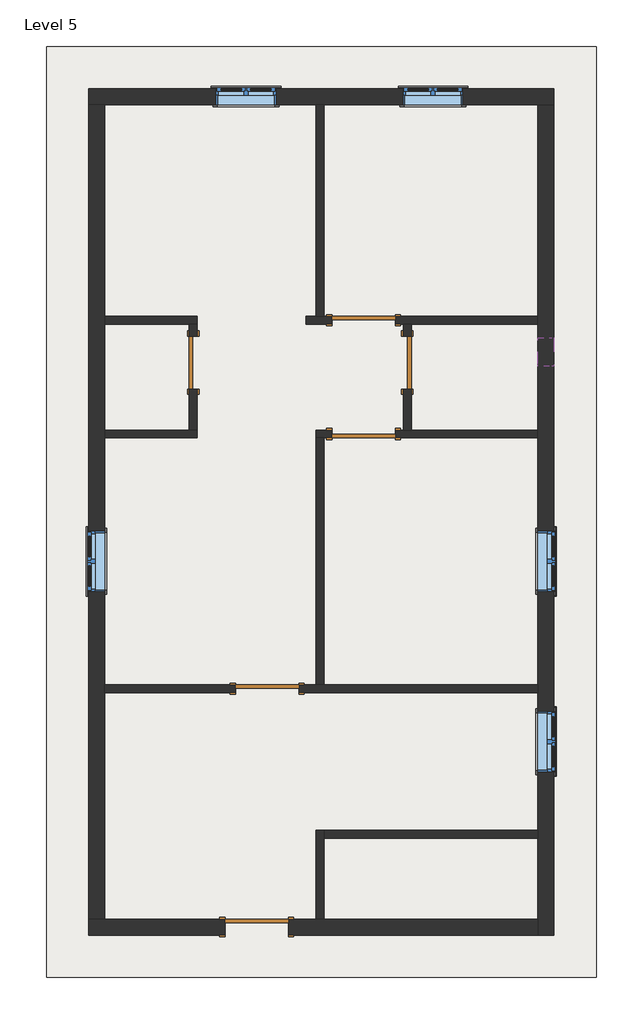
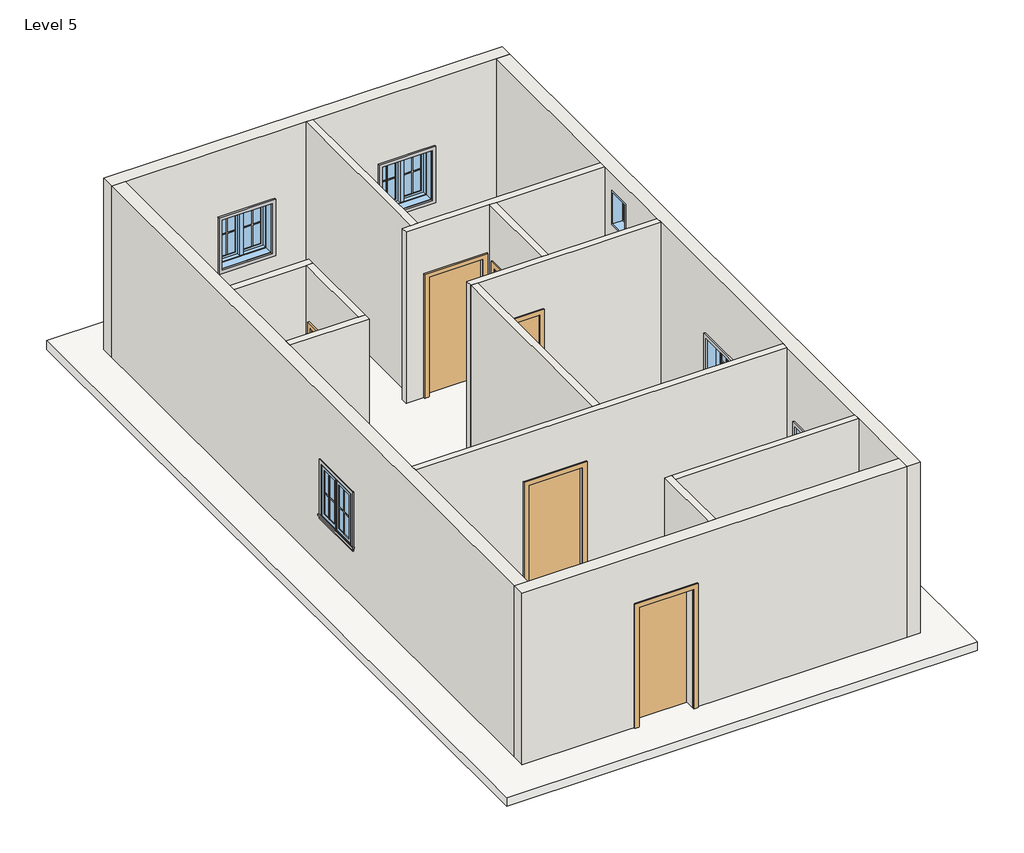
# One storey, incomplete: 20 proxies, 15 walls, 6 doors, 6 windows, 1 roof.
"""IFC4 building model written with IfcOpenShell, lengths in millimetres."""

from ifc_helpers import new_model, si_unit, frame, origin, place, context, project, spatial, polyline, outline, extrude, faceted_brep, transform, mapped, element, save
from components import muntin_pattern_2x2_muntin_pattern_2x2_b3fe6957, muntin_pattern_2x2_muntin_pattern_2x2_3e0ecaf2, trim_window_exterior_flat_with_sill_41619996, trim_window_interior_flat_picture_frame_51c85655, door_f2b275c1, door_d8f5dbb5, door_305aa2a5, door_e5f9f3c4, door_a90ba1ad, window_aa618e30, window_339605e1

model = new_model("IFC4")

# Units and contexts
model_context = context("Model", 3, world=origin())
ifc_project = project(units=[si_unit("LENGTHUNIT", "METRE", prefix="MILLI")], contexts=[model_context])

# Site, building, storey
site = spatial("IfcSite", under=ifc_project)
building = spatial("IfcBuilding", under=site)
storey = spatial("IfcBuildingStorey", under=building, Name="Level 5", Elevation=9601.2)

# Proxies
placement = place(None, origin())
muntin_pattern_2x2_muntin_pattern_2x2_shape = muntin_pattern_2x2_muntin_pattern_2x2_b3fe6957(model_context)
element("IfcBuildingElementProxy", 1, Name="Muntin Pattern_2x2 : Muntin Pattern_2x2", ObjectType="Muntin Pattern_2x2 : Muntin Pattern_2x2", at=placement, inside=storey, context=model_context, shape_type="MappedRepresentation", body=[
    mapped(muntin_pattern_2x2_muntin_pattern_2x2_shape, transform((-2560.703247, 6624.6685985, 10585.45), x_axis=(1.0, 0.0, 0.0), y_axis=(0.0, 1.0, 0.0), z_axis=(0.0, 0.0, 1.0))),
])
element("IfcBuildingElementProxy", 2, Name="Muntin Pattern_2x2 : Muntin Pattern_2x2", ObjectType="Muntin Pattern_2x2 : Muntin Pattern_2x2", at=placement, inside=storey, context=model_context, shape_type="MappedRepresentation", body=[
    mapped(muntin_pattern_2x2_muntin_pattern_2x2_shape, transform((134.871753, 6624.6685985, 10585.45), x_axis=(1.0, 0.0, 0.0), y_axis=(0.0, 1.0, 0.0), z_axis=(0.0, 0.0, 1.0))),
])
element("IfcBuildingElementProxy", 3, Name="Muntin Pattern_2x2 : Muntin Pattern_2x2", ObjectType="Muntin Pattern_2x2 : Muntin Pattern_2x2", at=placement, inside=storey, context=model_context, shape_type="MappedRepresentation", body=[
    mapped(muntin_pattern_2x2_muntin_pattern_2x2_shape, transform((2082.734253, 41.3060985, 10585.45), x_axis=(0.0, -1.0, 0.0), y_axis=(1.0, 0.0, 0.0), z_axis=(0.0, 0.0, 1.0))),
])
element("IfcBuildingElementProxy", 4, Name="Muntin Pattern_2x2 : Muntin Pattern_2x2", ObjectType="Muntin Pattern_2x2 : Muntin Pattern_2x2", at=placement, inside=storey, context=model_context, shape_type="MappedRepresentation", body=[
    mapped(muntin_pattern_2x2_muntin_pattern_2x2_shape, transform((-4603.815747, -387.3189015, 10585.45), x_axis=(0.0, 1.0, 0.0), y_axis=(-1.0, 0.0, 0.0), z_axis=(0.0, 0.0, 1.0))),
])
element("IfcBuildingElementProxy", 5, Name="Muntin Pattern_2x2 : Muntin Pattern_2x2", ObjectType="Muntin Pattern_2x2 : Muntin Pattern_2x2", at=placement, inside=storey, context=model_context, shape_type="MappedRepresentation", body=[
    mapped(muntin_pattern_2x2_muntin_pattern_2x2_shape, transform((2082.734253, -2555.8439015, 10585.45), x_axis=(0.0, -1.0, 0.0), y_axis=(1.0, 0.0, 0.0), z_axis=(0.0, 0.0, 1.0))),
])
muntin_pattern_2x2_muntin_pattern_2x2_2_shape = muntin_pattern_2x2_muntin_pattern_2x2_3e0ecaf2(model_context)
element("IfcBuildingElementProxy", 6, Name="Muntin Pattern_2x2 : Muntin Pattern_2x2", ObjectType="Muntin Pattern_2x2 : Muntin Pattern_2x2", at=placement, inside=storey, context=model_context, shape_type="MappedRepresentation", body=[
    mapped(muntin_pattern_2x2_muntin_pattern_2x2_2_shape, transform((-2132.078247, 6624.6685985, 10585.45), x_axis=(-1.0, 0.0, 0.0), y_axis=(0.0, -1.0, 0.0), z_axis=(0.0, 0.0, 1.0))),
])
element("IfcBuildingElementProxy", 7, Name="Muntin Pattern_2x2 : Muntin Pattern_2x2", ObjectType="Muntin Pattern_2x2 : Muntin Pattern_2x2", at=placement, inside=storey, context=model_context, shape_type="MappedRepresentation", body=[
    mapped(muntin_pattern_2x2_muntin_pattern_2x2_2_shape, transform((563.496753, 6624.6685985, 10585.45), x_axis=(-1.0, 0.0, 0.0), y_axis=(0.0, -1.0, 0.0), z_axis=(0.0, 0.0, 1.0))),
])
element("IfcBuildingElementProxy", 8, Name="Muntin Pattern_2x2 : Muntin Pattern_2x2", ObjectType="Muntin Pattern_2x2 : Muntin Pattern_2x2", at=placement, inside=storey, context=model_context, shape_type="MappedRepresentation", body=[
    mapped(muntin_pattern_2x2_muntin_pattern_2x2_2_shape, transform((2082.734253, -387.3189015, 10585.45), x_axis=(0.0, 1.0, 0.0), y_axis=(-1.0, 0.0, 0.0), z_axis=(0.0, 0.0, 1.0))),
])
element("IfcBuildingElementProxy", 9, Name="Muntin Pattern_2x2 : Muntin Pattern_2x2", ObjectType="Muntin Pattern_2x2 : Muntin Pattern_2x2", at=placement, inside=storey, context=model_context, shape_type="MappedRepresentation", body=[
    mapped(muntin_pattern_2x2_muntin_pattern_2x2_2_shape, transform((-4603.815747, 41.3060985, 10585.45), x_axis=(0.0, -1.0, 0.0), y_axis=(1.0, 0.0, 0.0), z_axis=(0.0, 0.0, 1.0))),
])
element("IfcBuildingElementProxy", 10, Name="Muntin Pattern_2x2 : Muntin Pattern_2x2", ObjectType="Muntin Pattern_2x2 : Muntin Pattern_2x2", at=placement, inside=storey, context=model_context, shape_type="MappedRepresentation", body=[
    mapped(muntin_pattern_2x2_muntin_pattern_2x2_2_shape, transform((2082.734253, -2984.4689015, 10585.45), x_axis=(0.0, 1.0, 0.0), y_axis=(-1.0, 0.0, 0.0), z_axis=(0.0, 0.0, 1.0))),
])
trim_window_exterior_flat_with_sill_shape = trim_window_exterior_flat_with_sill_41619996(model_context)
element("IfcBuildingElementProxy", 11, Name="Trim-Window-Exterior-Flat : with Sill", ObjectType="Trim-Window-Exterior-Flat : with Sill", at=placement, inside=storey, context=model_context, shape_type="MappedRepresentation", body=[
    mapped(trim_window_exterior_flat_with_sill_shape, transform((-2346.390747, 6634.1935985, 11430.0), x_axis=(-1.0, 0.0, 0.0), y_axis=(0.0, 0.0, 1.0), z_axis=(0.0, 1.0, 0.0))),
])
element("IfcBuildingElementProxy", 12, Name="Trim-Window-Exterior-Flat : with Sill", ObjectType="Trim-Window-Exterior-Flat : with Sill", at=placement, inside=storey, context=model_context, shape_type="MappedRepresentation", body=[
    mapped(trim_window_exterior_flat_with_sill_shape, transform((349.184253, 6634.1935985, 11430.0), x_axis=(-1.0, 0.0, 0.0), y_axis=(0.0, 0.0, 1.0), z_axis=(0.0, 1.0, 0.0))),
])
element("IfcBuildingElementProxy", 13, Name="Trim-Window-Exterior-Flat : with Sill", ObjectType="Trim-Window-Exterior-Flat : with Sill", at=placement, inside=storey, context=model_context, shape_type="MappedRepresentation", body=[
    mapped(trim_window_exterior_flat_with_sill_shape, transform((2092.259253, -173.0064015, 11430.0), x_axis=(0.0, 1.0, 0.0), y_axis=(0.0, 0.0, 1.0), z_axis=(1.0, 0.0, 0.0))),
])
element("IfcBuildingElementProxy", 14, Name="Trim-Window-Exterior-Flat : with Sill", ObjectType="Trim-Window-Exterior-Flat : with Sill", at=placement, inside=storey, context=model_context, shape_type="MappedRepresentation", body=[
    mapped(trim_window_exterior_flat_with_sill_shape, transform((-4613.340747, -173.0064015, 11430.0), x_axis=(0.0, -1.0, 0.0), y_axis=(0.0, 0.0, 1.0), z_axis=(-1.0, 0.0, 0.0))),
])
element("IfcBuildingElementProxy", 15, Name="Trim-Window-Exterior-Flat : with Sill", ObjectType="Trim-Window-Exterior-Flat : with Sill", at=placement, inside=storey, context=model_context, shape_type="MappedRepresentation", body=[
    mapped(trim_window_exterior_flat_with_sill_shape, transform((2092.259253, -2770.1564015, 11430.0), x_axis=(0.0, 1.0, 0.0), y_axis=(0.0, 0.0, 1.0), z_axis=(1.0, 0.0, 0.0))),
])
trim_window_interior_flat_picture_frame_shape = trim_window_interior_flat_picture_frame_51c85655(model_context)
element("IfcBuildingElementProxy", 16, Name="Trim-Window-Interior-Flat : Picture Frame", ObjectType="Trim-Window-Interior-Flat : Picture Frame", at=placement, inside=storey, context=model_context, shape_type="MappedRepresentation", body=[
    mapped(trim_window_interior_flat_picture_frame_shape, transform((-2346.390747, 6405.5935985, 11430.0), x_axis=(1.0, 0.0, 0.0), y_axis=(0.0, 0.0, 1.0), z_axis=(0.0, -1.0, 0.0))),
])
element("IfcBuildingElementProxy", 17, Name="Trim-Window-Interior-Flat : Picture Frame", ObjectType="Trim-Window-Interior-Flat : Picture Frame", at=placement, inside=storey, context=model_context, shape_type="MappedRepresentation", body=[
    mapped(trim_window_interior_flat_picture_frame_shape, transform((349.184253, 6405.5935985, 11430.0), x_axis=(1.0, 0.0, 0.0), y_axis=(0.0, 0.0, 1.0), z_axis=(0.0, -1.0, 0.0))),
])
element("IfcBuildingElementProxy", 18, Name="Trim-Window-Interior-Flat : Picture Frame", ObjectType="Trim-Window-Interior-Flat : Picture Frame", at=placement, inside=storey, context=model_context, shape_type="MappedRepresentation", body=[
    mapped(trim_window_interior_flat_picture_frame_shape, transform((1863.659253, -173.0064015, 11430.0), x_axis=(0.0, -1.0, 0.0), y_axis=(0.0, 0.0, 1.0), z_axis=(-1.0, 0.0, 0.0))),
])
element("IfcBuildingElementProxy", 19, Name="Trim-Window-Interior-Flat : Picture Frame", ObjectType="Trim-Window-Interior-Flat : Picture Frame", at=placement, inside=storey, context=model_context, shape_type="MappedRepresentation", body=[
    mapped(trim_window_interior_flat_picture_frame_shape, transform((-4384.740747, -173.0064015, 11430.0), x_axis=(0.0, 1.0, 0.0), y_axis=(0.0, 0.0, 1.0), z_axis=(1.0, 0.0, 0.0))),
])
element("IfcBuildingElementProxy", 20, Name="Trim-Window-Interior-Flat : Picture Frame", ObjectType="Trim-Window-Interior-Flat : Picture Frame", at=placement, inside=storey, context=model_context, shape_type="MappedRepresentation", body=[
    mapped(trim_window_interior_flat_picture_frame_shape, transform((1863.659253, -2770.1564015, 11430.0), x_axis=(0.0, -1.0, 0.0), y_axis=(0.0, 0.0, 1.0), z_axis=(-1.0, 0.0, 0.0))),
])

# Doors
door_shape = door_f2b275c1(model_context)
element("IfcDoor", 21, ObjectType="Single-Flush : 30\" x 80\"", at=placement, inside=storey, context=model_context, shape_type="MappedRepresentation", body=[
    mapped(door_shape, transform((-22.290747, 2690.8435985, 9601.2), x_axis=(0.0, 1.0, 0.0), y_axis=(-1.0, 0.0, 0.0), z_axis=(0.0, 0.0, 1.0))),
])
door_2_shape = door_d8f5dbb5(model_context)
element("IfcDoor", 22, ObjectType="Single-Flush : 30\" x 80\"", at=placement, inside=storey, context=model_context, shape_type="MappedRepresentation", body=[
    mapped(door_2_shape, transform((-3108.390747, 2690.8435985, 9601.2), x_axis=(0.0, 1.0, 0.0), y_axis=(-1.0, 0.0, 0.0), z_axis=(0.0, 0.0, 1.0))),
])
door_3_shape = door_305aa2a5(model_context)
element("IfcDoor", 23, ObjectType="Single-Flush : 36\" x 84\"", at=placement, inside=storey, context=model_context, shape_type="MappedRepresentation", body=[
    mapped(door_3_shape, transform((-650.940747, 3300.4435985, 9601.2), x_axis=(-1.0, 0.0, 0.0), y_axis=(0.0, -1.0, 0.0), z_axis=(0.0, 0.0, 1.0))),
])
door_4_shape = door_e5f9f3c4(model_context)
element("IfcDoor", 24, ObjectType="Single-Flush : 36\" x 84\"", at=placement, inside=storey, context=model_context, shape_type="MappedRepresentation", body=[
    mapped(door_4_shape, transform((-2041.590747, -2008.1564015, 9601.2), x_axis=(1.0, 0.0, 0.0), y_axis=(0.0, 1.0, 0.0), z_axis=(0.0, 0.0, 1.0))),
])
element("IfcDoor", 25, ObjectType="Single-Flush : 36\" x 84\"", at=placement, inside=storey, context=model_context, shape_type="MappedRepresentation", body=[
    mapped(door_4_shape, transform((-650.940747, 1662.1435985, 9601.2), x_axis=(-1.0, 0.0, 0.0), y_axis=(0.0, -1.0, 0.0), z_axis=(0.0, 0.0, 1.0))),
])
door_5_shape = door_a90ba1ad(model_context)
element("IfcDoor", 26, ObjectType="Single-Flush : 36\" x 84\"", at=placement, inside=storey, context=model_context, shape_type="MappedRepresentation", body=[
    mapped(door_5_shape, transform((-2193.990747, -5443.5064015, 9601.2), x_axis=(-1.0, 0.0, 0.0), y_axis=(0.0, -1.0, 0.0), z_axis=(0.0, 0.0, 1.0))),
])

# Roof
element("IfcRoof", 27, ObjectType="Generic - 12\"", at=placement, inside=storey, context=model_context, shape_type="SweptSolid", body=[
    extrude(outline(polyline([(-5222.940747, 7243.7935985), (2701.859253, 7243.7935985), (2701.859253, -6167.4064015), (-5222.940747, -6167.4064015), (-5222.940747, 7243.7935985)])), frame((0.0, 0.0, 9448.8), z_axis=(0.0, 0.0, 1.0), x_axis=(1.0, 0.0, 0.0)), (0.0, 0.0, 1.0), 152.4),
])

# Walls
element("IfcWall", 28, ObjectType="WALL4.5\"", at=placement, inside=storey, context=model_context, shape_type="Brep", body=[
    faceted_brep([(-4384.740747, 3243.2935985, 9601.2), (-3165.540747, 3243.2935985, 9601.2), (-3051.240747, 3243.2935985, 9601.2), (-3051.240747, 3243.2935985, 12649.2), (-3165.540747, 3243.2935985, 12649.2), (-4384.740747, 3243.2935985, 12649.2), (-4384.740747, 3357.5935985, 9601.2), (-4384.740747, 3357.5935985, 12649.2), (-3051.240747, 3357.5935985, 12649.2), (-3051.240747, 3357.5935985, 9601.2)], [[[0, 1, 2, 3, 4, 5]], [[6, 7, 8, 9]], [[2, 1, 0, 6, 9]], [[0, 5, 7, 6]], [[3, 2, 9, 8]], [[5, 4, 3, 8, 7]]]),
])
element("IfcWall", 29, ObjectType="WALL4.5\"", at=placement, inside=storey, context=model_context, shape_type="Brep", body=[
    faceted_brep([(-4384.740747, 1604.9935985, 9601.2), (-3051.240747, 1604.9935985, 9601.2), (-3051.240747, 1604.9935985, 12649.2), (-4384.740747, 1604.9935985, 12649.2), (-4384.740747, 1719.2935985, 9601.2), (-4384.740747, 1719.2935985, 12649.2), (-3165.540747, 1719.2935985, 12649.2), (-3051.240747, 1719.2935985, 12649.2), (-3051.240747, 1719.2935985, 9601.2), (-3165.540747, 1719.2935985, 9601.2)], [[[0, 1, 2, 3]], [[4, 5, 6, 7, 8, 9]], [[1, 0, 4, 9, 8]], [[0, 3, 5, 4]], [[2, 1, 8, 7]], [[3, 2, 7, 6, 5]]]),
])
element("IfcWall", 30, ObjectType="WALL4.5\"", at=placement, inside=storey, context=model_context, shape_type="SweptSolid", body=[
    extrude(outline(polyline([(3243.2935985, 9601.2), (3071.8435985, 9601.2), (3071.8435985, 11633.2), (2309.8435985, 11633.2), (2309.8435985, 9601.2), (1719.2935985, 9601.2), (1719.2935985, 12649.2), (3243.2935985, 12649.2), (3243.2935985, 9601.2)])), frame((-3165.540747, 0.0, 0.0), z_axis=(1.0, 0.0, 0.0), x_axis=(0.0, 1.0, 0.0)), (0.0, 0.0, 1.0), 114.3),
])
element("IfcWall", 31, ObjectType="WALL4.5\"", at=placement, inside=storey, context=model_context, shape_type="SweptSolid", body=[
    extrude(outline(polyline([(-1336.740747, 3357.5935985), (-1336.740747, 6405.5935985), (-1222.440747, 6405.5935985), (-1222.440747, 3357.5935985), (-1336.740747, 3357.5935985)])), frame((0.0, 0.0, 9601.2), z_axis=(0.0, 0.0, 1.0), x_axis=(1.0, 0.0, 0.0)), (0.0, 0.0, 1.0), 3048.0),
])
element("IfcWall", 32, ObjectType="WALL4.5\"", at=placement, inside=storey, context=model_context, shape_type="Brep", body=[
    faceted_brep([(-1481.7019184, 3243.2935985, 9601.2), (-1108.140747, 3243.2935985, 9601.2), (-1108.140747, 3243.2935985, 11734.8), (-193.740747, 3243.2935985, 11734.8), (-193.740747, 3243.2935985, 9601.2), (-79.440747, 3243.2935985, 9601.2), (34.859253, 3243.2935985, 9601.2), (1863.659253, 3243.2935985, 9601.2), (1863.659253, 3243.2935985, 12649.2), (34.859253, 3243.2935985, 12649.2), (-79.440747, 3243.2935985, 12649.2), (-1481.7019184, 3243.2935985, 12649.2), (-1108.140747, 3357.5935985, 11734.8), (-1108.140747, 3357.5935985, 9601.2), (-1222.440747, 3357.5935985, 9601.2), (-1336.740747, 3357.5935985, 9601.2), (-1481.7019184, 3357.5935985, 9601.2), (-1481.7019184, 3357.5935985, 12649.2), (-1336.740747, 3357.5935985, 12649.2), (-1222.440747, 3357.5935985, 12649.2), (1863.659253, 3357.5935985, 12649.2), (1863.659253, 3357.5935985, 9601.2), (-193.740747, 3357.5935985, 9601.2), (-193.740747, 3357.5935985, 11734.8)], [[[0, 1, 2, 3, 4, 5, 6, 7, 8, 9, 10, 11]], [[12, 13, 14, 15, 16, 17, 18, 19, 20, 21, 22, 23]], [[22, 21, 7, 6, 5, 4]], [[16, 15, 14, 13, 1, 0]], [[0, 11, 17, 16]], [[8, 7, 21, 20]], [[2, 1, 13, 12]], [[3, 2, 12, 23]], [[4, 3, 23, 22]], [[11, 10, 9, 8, 20, 19, 18, 17]]]),
])
element("IfcWall", 33, ObjectType="WALL4.5\"", at=placement, inside=storey, context=model_context, shape_type="SweptSolid", body=[
    extrude(outline(polyline([(3243.2935985, 9601.2), (3071.8435985, 9601.2), (3071.8435985, 11633.2), (2309.8435985, 11633.2), (2309.8435985, 9601.2), (1719.2935985, 9601.2), (1719.2935985, 12649.2), (3243.2935985, 12649.2), (3243.2935985, 9601.2)])), frame((-79.440747, 0.0, 0.0), z_axis=(1.0, 0.0, 0.0), x_axis=(0.0, 1.0, 0.0)), (0.0, 0.0, 1.0), 114.3),
])
element("IfcWall", 34, ObjectType="WALL4.5\"", at=placement, inside=storey, context=model_context, shape_type="Brep", body=[
    faceted_brep([(-1108.140747, 1719.2935985, 11734.8), (-1108.140747, 1719.2935985, 9601.2), (-1336.740747, 1719.2935985, 9601.2), (-1336.740747, 1719.2935985, 12649.2), (-79.440747, 1719.2935985, 12649.2), (34.859253, 1719.2935985, 12649.2), (1863.659253, 1719.2935985, 12649.2), (1863.659253, 1719.2935985, 9601.2), (34.859253, 1719.2935985, 9601.2), (-79.440747, 1719.2935985, 9601.2), (-193.740747, 1719.2935985, 9601.2), (-193.740747, 1719.2935985, 11734.8), (-1336.740747, 1604.9935985, 9601.2), (-1222.440747, 1604.9935985, 9601.2), (-1108.140747, 1604.9935985, 9601.2), (-1108.140747, 1604.9935985, 11734.8), (-193.740747, 1604.9935985, 11734.8), (-193.740747, 1604.9935985, 9601.2), (1863.659253, 1604.9935985, 9601.2), (1863.659253, 1604.9935985, 12649.2), (-1222.440747, 1604.9935985, 12649.2), (-1336.740747, 1604.9935985, 12649.2)], [[[0, 1, 2, 3, 4, 5, 6, 7, 8, 9, 10, 11]], [[12, 13, 14, 15, 16, 17, 18, 19, 20, 21]], [[2, 1, 14, 13, 12]], [[10, 9, 8, 7, 18, 17]], [[7, 6, 19, 18]], [[3, 2, 12, 21]], [[15, 14, 1, 0]], [[16, 15, 0, 11]], [[17, 16, 11, 10]], [[6, 5, 4, 3, 21, 20, 19]]]),
])
element("IfcWall", 35, ObjectType="WALL4.5\"", at=placement, inside=storey, context=model_context, shape_type="SweptSolid", body=[
    extrude(outline(polyline([(-1336.740747, -1951.0064015), (-1336.740747, 1604.9935985), (-1222.440747, 1604.9935985), (-1222.440747, -1951.0064015), (-1336.740747, -1951.0064015)])), frame((0.0, 0.0, 9601.2), z_axis=(0.0, 0.0, 1.0), x_axis=(1.0, 0.0, 0.0)), (0.0, 0.0, 1.0), 3048.0),
])
element("IfcWall", 36, ObjectType="WALL4.5\"", at=placement, inside=storey, context=model_context, shape_type="Brep", body=[
    faceted_brep([(-1584.390747, -2065.3064015, 11734.8), (-1584.390747, -2065.3064015, 9601.2), (1863.659253, -2065.3064015, 9601.2), (1863.659253, -2065.3064015, 12649.2), (-4384.740747, -2065.3064015, 12649.2), (-4384.740747, -2065.3064015, 9601.2), (-2498.790747, -2065.3064015, 9601.2), (-2498.790747, -2065.3064015, 11734.8), (1863.659253, -1951.0064015, 9601.2), (-1222.440747, -1951.0064015, 9601.2), (-1336.740747, -1951.0064015, 9601.2), (-1584.390747, -1951.0064015, 9601.2), (-1584.390747, -1951.0064015, 11734.8), (-2498.790747, -1951.0064015, 11734.8), (-2498.790747, -1951.0064015, 9601.2), (-4384.740747, -1951.0064015, 9601.2), (-4384.740747, -1951.0064015, 12649.2), (-1336.740747, -1951.0064015, 12649.2), (-1222.440747, -1951.0064015, 12649.2), (1863.659253, -1951.0064015, 12649.2)], [[[0, 1, 2, 3, 4, 5, 6, 7]], [[8, 9, 10, 11, 12, 13, 14, 15, 16, 17, 18, 19]], [[6, 5, 15, 14]], [[2, 1, 11, 10, 9, 8]], [[3, 2, 8, 19]], [[5, 4, 16, 15]], [[12, 11, 1, 0]], [[13, 12, 0, 7]], [[14, 13, 7, 6]], [[4, 3, 19, 18, 17, 16]]]),
])
element("IfcWall", 37, ObjectType="WALL4.5\"", at=placement, inside=storey, context=model_context, shape_type="Brep", body=[
    faceted_brep([(-1222.440747, -5329.2064015, 9601.2), (-1222.440747, -4160.8064015, 9601.2), (-1222.440747, -4046.5064015, 9601.2), (-1222.440747, -4046.5064015, 12649.2), (-1222.440747, -4160.8064015, 12649.2), (-1222.440747, -5329.2064015, 12649.2), (-1336.740747, -5329.2064015, 9601.2), (-1336.740747, -5329.2064015, 12649.2), (-1336.740747, -4046.5064015, 12649.2), (-1336.740747, -4046.5064015, 9601.2)], [[[0, 1, 2, 3, 4, 5]], [[6, 7, 8, 9]], [[2, 1, 0, 6, 9]], [[0, 5, 7, 6]], [[3, 2, 9, 8]], [[5, 4, 3, 8, 7]]]),
])
element("IfcWall", 38, ObjectType="WALL4.5\"", at=placement, inside=storey, context=model_context, shape_type="SweptSolid", body=[
    extrude(outline(polyline([(1863.659253, -4160.8064015), (-1222.440747, -4160.8064015), (-1222.440747, -4046.5064015), (1863.659253, -4046.5064015), (1863.659253, -4160.8064015)])), frame((0.0, 0.0, 9601.2), z_axis=(0.0, 0.0, 1.0), x_axis=(1.0, 0.0, 0.0)), (0.0, 0.0, 1.0), 3048.0),
])
element("IfcWall", 39, ObjectType="WALL9\"", at=placement, inside=storey, context=model_context, shape_type="Brep", body=[
    faceted_brep([(-4613.340747, 6405.5935985, 9601.2), (-4384.740747, 6405.5935985, 9601.2), (-1336.740747, 6405.5935985, 9601.2), (-1222.440747, 6405.5935985, 9601.2), (1863.659253, 6405.5935985, 9601.2), (2092.259253, 6405.5935985, 9601.2), (2092.259253, 6405.5935985, 12649.2), (1863.659253, 6405.5935985, 12649.2), (-1222.440747, 6405.5935985, 12649.2), (-1336.740747, 6405.5935985, 12649.2), (-4384.740747, 6405.5935985, 12649.2), (-4613.340747, 6405.5935985, 12649.2), (-1914.590747, 6405.5935985, 11430.0), (-1914.590747, 6405.5935985, 10515.6), (-2778.190747, 6405.5935985, 10515.6), (-2778.190747, 6405.5935985, 11430.0), (780.984253, 6405.5935985, 11430.0), (780.984253, 6405.5935985, 10515.6), (-82.615747, 6405.5935985, 10515.6), (-82.615747, 6405.5935985, 11430.0), (-4613.340747, 6634.1935985, 9601.2), (-4613.340747, 6634.1935985, 12649.2), (2092.259253, 6634.1935985, 12649.2), (2092.259253, 6634.1935985, 9601.2), (-1914.590747, 6634.1935985, 11430.0), (-2778.190747, 6634.1935985, 11430.0), (-2778.190747, 6634.1935985, 10515.6), (-1914.590747, 6634.1935985, 10515.6), (780.984253, 6634.1935985, 11430.0), (-82.615747, 6634.1935985, 11430.0), (-82.615747, 6634.1935985, 10515.6), (780.984253, 6634.1935985, 10515.6)], [[[0, 1, 2, 3, 4, 5, 6, 7, 8, 9, 10, 11], [12, 13, 14, 15], [16, 17, 18, 19]], [[20, 21, 22, 23], [24, 25, 26, 27], [28, 29, 30, 31]], [[5, 4, 3, 2, 1, 0, 20, 23]], [[6, 5, 23, 22]], [[0, 11, 21, 20]], [[13, 12, 24, 27]], [[14, 13, 27, 26]], [[15, 14, 26, 25]], [[12, 15, 25, 24]], [[17, 16, 28, 31]], [[18, 17, 31, 30]], [[19, 18, 30, 29]], [[16, 19, 29, 28]], [[11, 10, 9, 8, 7, 6, 22, 21]]]),
])
element("IfcWall", 40, ObjectType="WALL9\"", at=placement, inside=storey, context=model_context, shape_type="Brep", body=[
    faceted_brep([(1863.659253, 6405.5935985, 9601.2), (1863.659253, 3357.5935985, 9601.2), (1863.659253, 3243.2935985, 9601.2), (1863.659253, 1719.2935985, 9601.2), (1863.659253, 1604.9935985, 9601.2), (1863.659253, -1951.0064015, 9601.2), (1863.659253, -2065.3064015, 9601.2), (1863.659253, -4046.5064015, 9601.2), (1863.659253, -4160.8064015, 9601.2), (1863.659253, -5329.2064015, 9601.2), (1863.659253, -5557.8064015, 9601.2), (1863.659253, -5557.8064015, 12649.2), (1863.659253, -5329.2064015, 12649.2), (1863.659253, -4160.8064015, 12649.2), (1863.659253, -4046.5064015, 12649.2), (1863.659253, -2065.3064015, 12649.2), (1863.659253, -1951.0064015, 12649.2), (1863.659253, 1604.9935985, 12649.2), (1863.659253, 1719.2935985, 12649.2), (1863.659253, 3243.2935985, 12649.2), (1863.659253, 3357.5935985, 12649.2), (1863.659253, 6405.5935985, 12649.2), (1863.659253, 2640.0435985, 12344.4), (1863.659253, 2640.0435985, 11734.8), (1863.659253, 3046.4435985, 11734.8), (1863.659253, 3046.4435985, 12344.4), (1863.659253, -604.8064015, 11430.0), (1863.659253, -604.8064015, 10515.6), (1863.659253, 258.7935985, 10515.6), (1863.659253, 258.7935985, 11430.0), (1863.659253, -3201.9564015, 11430.0), (1863.659253, -3201.9564015, 10515.6), (1863.659253, -2338.3564015, 10515.6), (1863.659253, -2338.3564015, 11430.0), (2092.259253, 6405.5935985, 9601.2), (2092.259253, 6405.5935985, 12649.2), (2092.259253, -5557.8064015, 12649.2), (2092.259253, -5557.8064015, 9601.2), (2092.259253, 2640.0435985, 12344.4), (2092.259253, 3046.4435985, 12344.4), (2092.259253, 3046.4435985, 11734.8), (2092.259253, 2640.0435985, 11734.8), (2092.259253, -604.8064015, 11430.0), (2092.259253, 258.7935985, 11430.0), (2092.259253, 258.7935985, 10515.6), (2092.259253, -604.8064015, 10515.6), (2092.259253, -3201.9564015, 11430.0), (2092.259253, -2338.3564015, 11430.0), (2092.259253, -2338.3564015, 10515.6), (2092.259253, -3201.9564015, 10515.6)], [[[0, 1, 2, 3, 4, 5, 6, 7, 8, 9, 10, 11, 12, 13, 14, 15, 16, 17, 18, 19, 20, 21], [22, 23, 24, 25], [26, 27, 28, 29], [30, 31, 32, 33]], [[34, 35, 36, 37], [38, 39, 40, 41], [42, 43, 44, 45], [46, 47, 48, 49]], [[10, 9, 8, 7, 6, 5, 4, 3, 2, 1, 0, 34, 37]], [[0, 21, 35, 34]], [[11, 10, 37, 36]], [[23, 22, 38, 41]], [[24, 23, 41, 40]], [[25, 24, 40, 39]], [[22, 25, 39, 38]], [[27, 26, 42, 45]], [[28, 27, 45, 44]], [[29, 28, 44, 43]], [[26, 29, 43, 42]], [[31, 30, 46, 49]], [[32, 31, 49, 48]], [[33, 32, 48, 47]], [[30, 33, 47, 46]], [[21, 20, 19, 18, 17, 16, 15, 14, 13, 12, 11, 36, 35]]]),
])
element("IfcWall", 41, ObjectType="WALL9\"", at=placement, inside=storey, context=model_context, shape_type="Brep", body=[
    faceted_brep([(-2651.190747, -5329.2064015, 11734.8), (-2651.190747, -5329.2064015, 9601.2), (-4384.740747, -5329.2064015, 9601.2), (-4613.340747, -5329.2064015, 9601.2), (-4613.340747, -5329.2064015, 12649.2), (-4384.740747, -5329.2064015, 12649.2), (-1336.740747, -5329.2064015, 12649.2), (-1222.440747, -5329.2064015, 12649.2), (1863.659253, -5329.2064015, 12649.2), (1863.659253, -5329.2064015, 9601.2), (-1222.440747, -5329.2064015, 9601.2), (-1336.740747, -5329.2064015, 9601.2), (-1736.790747, -5329.2064015, 9601.2), (-1736.790747, -5329.2064015, 11734.8), (-4613.340747, -5557.8064015, 9601.2), (-2651.190747, -5557.8064015, 9601.2), (-2651.190747, -5557.8064015, 11734.8), (-1736.790747, -5557.8064015, 11734.8), (-1736.790747, -5557.8064015, 9601.2), (1863.659253, -5557.8064015, 9601.2), (1863.659253, -5557.8064015, 12649.2), (-4613.340747, -5557.8064015, 12649.2)], [[[0, 1, 2, 3, 4, 5, 6, 7, 8, 9, 10, 11, 12, 13]], [[14, 15, 16, 17, 18, 19, 20, 21]], [[3, 2, 1, 15, 14]], [[12, 11, 10, 9, 19, 18]], [[9, 8, 20, 19]], [[4, 3, 14, 21]], [[16, 15, 1, 0]], [[17, 16, 0, 13]], [[18, 17, 13, 12]], [[8, 7, 6, 5, 4, 21, 20]]]),
])
element("IfcWall", 42, ObjectType="WALL9\"", at=placement, inside=storey, context=model_context, shape_type="Brep", body=[
    faceted_brep([(-4384.740747, -5329.2064015, 9601.2), (-4384.740747, -2065.3064015, 9601.2), (-4384.740747, -1951.0064015, 9601.2), (-4384.740747, 1604.9935985, 9601.2), (-4384.740747, 1719.2935985, 9601.2), (-4384.740747, 3243.2935985, 9601.2), (-4384.740747, 3357.5935985, 9601.2), (-4384.740747, 6405.5935985, 9601.2), (-4384.740747, 6405.5935985, 12649.2), (-4384.740747, 3357.5935985, 12649.2), (-4384.740747, 3243.2935985, 12649.2), (-4384.740747, 1719.2935985, 12649.2), (-4384.740747, 1604.9935985, 12649.2), (-4384.740747, -1951.0064015, 12649.2), (-4384.740747, -2065.3064015, 12649.2), (-4384.740747, -5329.2064015, 12649.2), (-4384.740747, 258.7935985, 11430.0), (-4384.740747, 258.7935985, 10515.6), (-4384.740747, -604.8064015, 10515.6), (-4384.740747, -604.8064015, 11430.0), (-4613.340747, -5329.2064015, 9601.2), (-4613.340747, -5329.2064015, 12649.2), (-4613.340747, 6405.5935985, 12649.2), (-4613.340747, 6405.5935985, 9601.2), (-4613.340747, 258.7935985, 11430.0), (-4613.340747, -604.8064015, 11430.0), (-4613.340747, -604.8064015, 10515.6), (-4613.340747, 258.7935985, 10515.6)], [[[0, 1, 2, 3, 4, 5, 6, 7, 8, 9, 10, 11, 12, 13, 14, 15], [16, 17, 18, 19]], [[20, 21, 22, 23], [24, 25, 26, 27]], [[7, 6, 5, 4, 3, 2, 1, 0, 20, 23]], [[8, 7, 23, 22]], [[0, 15, 21, 20]], [[17, 16, 24, 27]], [[18, 17, 27, 26]], [[19, 18, 26, 25]], [[16, 19, 25, 24]], [[15, 14, 13, 12, 11, 10, 9, 8, 22, 21]]]),
])

# Windows
window_shape = window_aa618e30(model_context)
element("IfcWindow", 43, ObjectType="Fixed : 16\" x 24\"", at=placement, inside=storey, context=model_context, shape_type="MappedRepresentation", body=[
    mapped(window_shape, transform((1977.959253, 2805.1435985, 10820.4), x_axis=(0.0, -1.0, 0.0), y_axis=(1.0, 0.0, 0.0), z_axis=(0.0, 0.0, 1.0))),
])
window_2_shape = window_339605e1(model_context)
element("IfcWindow", 44, ObjectType="Window-Casement-Double : 34\" x 36\"", at=placement, inside=storey, context=model_context, shape_type="MappedRepresentation", body=[
    mapped(window_2_shape, transform((-2346.390747, 6519.8935985, 9601.2), x_axis=(1.0, 0.0, 0.0), y_axis=(0.0, 1.0, 0.0), z_axis=(0.0, 0.0, 1.0))),
])
element("IfcWindow", 45, ObjectType="Window-Casement-Double : 34\" x 36\"", at=placement, inside=storey, context=model_context, shape_type="MappedRepresentation", body=[
    mapped(window_2_shape, transform((349.184253, 6519.8935985, 9601.2), x_axis=(1.0, 0.0, 0.0), y_axis=(0.0, 1.0, 0.0), z_axis=(0.0, 0.0, 1.0))),
])
element("IfcWindow", 46, ObjectType="Window-Casement-Double : 34\" x 36\"", at=placement, inside=storey, context=model_context, shape_type="MappedRepresentation", body=[
    mapped(window_2_shape, transform((1977.959253, -173.0064015, 9601.2), x_axis=(0.0, -1.0, 0.0), y_axis=(1.0, 0.0, 0.0), z_axis=(0.0, 0.0, 1.0))),
])
element("IfcWindow", 47, ObjectType="Window-Casement-Double : 34\" x 36\"", at=placement, inside=storey, context=model_context, shape_type="MappedRepresentation", body=[
    mapped(window_2_shape, transform((-4499.040747, -173.0064015, 9601.2), x_axis=(0.0, 1.0, 0.0), y_axis=(-1.0, 0.0, 0.0), z_axis=(0.0, 0.0, 1.0))),
])
element("IfcWindow", 48, ObjectType="Window-Casement-Double : 34\" x 36\"", at=placement, inside=storey, context=model_context, shape_type="MappedRepresentation", body=[
    mapped(window_2_shape, transform((1977.959253, -2770.1564015, 9601.2), x_axis=(0.0, -1.0, 0.0), y_axis=(1.0, 0.0, 0.0), z_axis=(0.0, 0.0, 1.0))),
])

save(model, "model.ifc")

# Revit data of these elements
# Type "Muntin Pattern_2x2 : Muntin Pattern_2x2"
#   Width [instance default] = 4' - 0"
#   Thickness = 0' - 0 1/2"
#   Height [instance default] = 4' - 0"
#   Distance = 0' - 0 3/4"
#   Interior Material [instance default] = none
#   Exterior Material [instance default] = none
#   Default Elevation = 0
# Type "Trim-Window-Exterior-Flat : with Sill"
#   Trim Width = 0' - 2 1/4"
#   Trim Thickness_Picture Frame = 0' - 1 1/4"
#   Trim Thickness_with Sill = 0' - 0 3/4"
#   Sill Thickness = 0' - 1 1/4"
#   Opening Width [instance default] = 2' - 0"
#   Opening Height [instance default] = 3' - 0"
#   Default Elevation = 4' - 0"
#   Sill = yes
#   Picture Frame = no
#   Trim Material [instance default] = none
# Type "Trim-Window-Interior-Flat : Picture Frame"
#   Trim Thickness_Picture Frame = 0' - 1 1/4"
#   Trim Width = 0' - 2 1/4"
#   Trim Thickness_with Sill = 0' - 0 3/4"
#   Sill Thickness = 0' - 1 1/4"
#   Opening Width [instance default] = 2' - 0"
#   Opening Height [instance default] = 3' - 0"
#   Default Elevation = 4' - 0"
#   Sill = no
#   Picture Frame = yes
#   Trim Material [instance default] = none
# Type "Single-Flush : 30\" x 80\""
#   Type Mark = "5"
#   Construction Type Id = "MDOOR"
#   Assembly Code = "C1020"
#   Analytic Construction = "Metal"
#   Thickness = 0' - 2"
#   Heat Transfer Coefficient (U) = 0.651978 BTU/(h·ft²·°F)
#   Height = 6' - 8"
#   Trim Projection Ext = 0' - 1"
#   Trim Projection Int = 0' - 1"
#   Trim Width = 0' - 3"
#   Width = 2' - 6"
#   Define Thermal Properties by = 1
#   Define Thermal Properties by = 1
#   Door Material = Door - Panel
#   Frame Material = Door - Frame
#   Visual Light Transmittance = 0
#   Solar Heat Gain Coefficient = 0
#   Function = (empty or 0)
#   Wall Closure = (empty or 0)
# Type "Single-Flush : 36\" x 84\""
#   Type Mark = "1"
#   Construction Type Id = "MDOOR"
#   Assembly Code = "C1020"
#   Analytic Construction = "Metal"
#   Thickness = 0' - 2"
#   Heat Transfer Coefficient (U) = 0.651978 BTU/(h·ft²·°F)
#   Height = 7' - 0"
#   Trim Projection Ext = 0' - 1"
#   Trim Projection Int = 0' - 1"
#   Trim Width = 0' - 3"
#   Width = 3' - 0"
#   Define Thermal Properties by = 1
#   Define Thermal Properties by = 1
#   Door Material = Door - Panel
#   Frame Material = Door - Frame
#   Visual Light Transmittance = 0
#   Solar Heat Gain Coefficient = 0
#   Function = (empty or 0)
#   Wall Closure = (empty or 0)
# Type "Generic - 12\""
#   Assembly Code = "B1020"
#   Layers, outside or top first: 0' - 6" no material (function 1)
# Type "WALL4.5\""
#   Assembly Code = "B2010"
#   Layers, outside or top first: 0' - 4 1/2" no material (function 1)
# Type "WALL9\""
#   Assembly Code = "B2010"
#   Layers, outside or top first: 0' - 9" no material (function 1)
# Type "Fixed : 16\" x 24\""
#   Type Mark = "4"
#   Construction Type Id = "GSP4R"
#   Assembly Code = "B2020100"
#   Analytic Construction = "1/8 in Pilkington single glazing"
#   Visual Light Transmittance = 0.9
#   Solar Heat Gain Coefficient = 0.78
#   Heat Transfer Coefficient (U) = 0.6496 BTU/(h·ft²·°F)
#   Height = 2' - 0"
#   Default Sill Height = 3' - 0"
#   Width = 1' - 4"
#   Window Inset = 0' - 0 3/4"
#   Define Thermal Properties by = 1
#   Define Thermal Properties by = 1
#   Glass Pane Material = Glass
#   Sash Material = Sash
#   Wall Closure = (empty or 0)
# Type "Window-Casement-Double : 34\" x 36\""
#   Type Mark = "14"
#   Fire Rating = "0.5h"
#   Assembly Code = "B2020100"
#   Analytic Construction = "Double glazing - domestic"
#   Frame Extension [instance default] = 0' - 0 1/4"
#   Window Inset [instance default] = 0' - 0"
#   Wall Thickness [instance default] = 0' - 6"
#   Interior Wall Closure [instance default] = 0' - 2 1/4"
#   Half Width = 1' - 5"
#   Visual Light Transmittance = 0.81
#   Thermal Resistance (R) = 1.8146 (h·ft²·°F)/BTU
#   Solar Heat Gain Coefficient = 0.76
#   Rough Width = 2' - 10 1/2"
#   Rough Height = 3' - 0 1/2"
#   Height = 3' - 0"
#   Heat Transfer Coefficient (U) = 0.5511 BTU/(h·ft²·°F)
#   Exterior Wall Closure [instance default] = 0' - 1 1/4"
#   Extension Jamb [instance default] = 0' - 2 1/4"
#   Default Sill Height = 3' - 0"
#   Width = 2' - 10"
#   Define Thermal Properties by = 0
#   Muntin Visibility = yes
#   Interior Trim Visibility [instance default] = yes
#   Exterior Trim Visibility [instance default] = yes
#   Extension Jamb Visibility [instance default] = yes
#   Interior Trim Material = Wood - Stained
#   Muntin Pattern = Muntin Pattern_2x2 : Muntin Pattern_2x2
#   Interior Trim = Trim-Window-Interior-Flat : Picture Frame
#   Interior Frame Material = Wood - Stained
#   Glass Panel Material = Glass
#   Exterior Trim Material = Clad - White
#   Exterior Trim = Trim-Window-Exterior-Flat : with Sill
#   Exterior Frame Material = Clad - White
#   Wall Closure = (empty or 0)
# Elements 1, 2, 3, 4, 5, 6, 7, 8, 9, 10 (IfcBuildingElementProxy, "Muntin Pattern_2x2 : Muntin Pattern_2x2")
#   Width = 0' - 11 5/8"
#   Height = 2' - 6 1/2"
#   Interior Material = Wood - Stained
#   Exterior Material = Clad - White
#   Phase Created = New Construction
#   Materials on its faces: "Clad - White", "Wood - Stained"
# Elements 11, 12, 13, 14, 15 (IfcBuildingElementProxy, "Trim-Window-Exterior-Flat : with Sill")
#   Opening Width = 2' - 10"
#   Opening Height = 3' - 0"
#   Trim Material = Clad - White
#   Phase Created = New Construction
#   Materials on its faces: "Clad - White"
# Elements 16, 17, 18, 19, 20 (IfcBuildingElementProxy, "Trim-Window-Interior-Flat : Picture Frame")
#   Opening Width = 2' - 10"
#   Opening Height = 3' - 0"
#   Trim Material = Wood - Stained
#   Phase Created = New Construction
#   Materials on its faces: "Wood - Stained"
# Elements 21, 22 (IfcDoor, "Single-Flush : 30\" x 80\"")
#   Phase Created = New Construction
#   Materials on its faces: "Door - Frame", "Door - Panel"
# Elements 23, 24, 25, 26 (IfcDoor, "Single-Flush : 36\" x 84\"")
#   Phase Created = New Construction
#   Materials on its faces: "Door - Frame", "Door - Panel"
# Element 27 (IfcRoof, "Generic - 12\"")
#   built-in parameter 1001705 = 31.5 (stored number, unit not read)
#   built-in parameter 1001701 = -0.5 (stored number, unit not read)
#   built-in parameter 1001710 = 33615
#   Phase Created = New Construction
#   Materials on its faces: "Default Roof", "Door - Panel"
# Elements 28, 29, 30, 31, 32, 33, 34, 35, 36, 37, 38 (IfcWall, "WALL4.5\"")
#   Top Offset = 0' - 0"
#   Base Offset = 0' - 0"
#   Unconnected Height = 10' - 0"
#   wall height = 10' - 0"
#   Phase Created = New Construction
#   Base Constraint = Level 5
#   Materials on its faces: "Default Wall"
# Elements 39, 40, 41, 42 (IfcWall, "WALL9\"")
#   Top Offset = 0' - 0"
#   Base Offset = 0' - 0"
#   Unconnected Height = 10' - 0"
#   wall height = 10' - 0"
#   Phase Created = New Construction
#   Base Constraint = Level 5
#   Materials on its faces: "Default Wall", "Door - Panel"
# Element 43 (IfcWindow, "Fixed : 16\" x 24\"")
#   Mark = "19"
#   Phase Created = New Construction
#   Materials on its faces: "Sash", "Glass"
# Element 44 (IfcWindow, "Window-Casement-Double : 34\" x 36\"")
#   Mark = "20"
#   Window Inset = 0' - 0"
#   Interior Wall Closure = 0' - 2 1/4"
#   Frame Extension = 0' - 0 1/4"
#   Exterior Wall Closure = 0' - 1 1/4"
#   Interior Trim Visibility = yes
#   Exterior Trim Visibility = yes
#   Phase Created = New Construction
#   Materials on its faces: "Wood - Stained", "Glass", "Clad - White"
# Element 45 (IfcWindow, "Window-Casement-Double : 34\" x 36\"")
#   Mark = "21"
#   Window Inset = 0' - 0"
#   Interior Wall Closure = 0' - 2 1/4"
#   Frame Extension = 0' - 0 1/4"
#   Exterior Wall Closure = 0' - 1 1/4"
#   Interior Trim Visibility = yes
#   Exterior Trim Visibility = yes
#   Phase Created = New Construction
#   Materials on its faces: "Wood - Stained", "Glass", "Clad - White"
# Element 46 (IfcWindow, "Window-Casement-Double : 34\" x 36\"")
#   Mark = "22"
#   Window Inset = 0' - 0"
#   Interior Wall Closure = 0' - 2 1/4"
#   Frame Extension = 0' - 0 1/4"
#   Exterior Wall Closure = 0' - 1 1/4"
#   Interior Trim Visibility = yes
#   Exterior Trim Visibility = yes
#   Phase Created = New Construction
#   Materials on its faces: "Wood - Stained", "Glass", "Clad - White"
# Element 47 (IfcWindow, "Window-Casement-Double : 34\" x 36\"")
#   Mark = "23"
#   Window Inset = 0' - 0"
#   Interior Wall Closure = 0' - 2 1/4"
#   Frame Extension = 0' - 0 1/4"
#   Exterior Wall Closure = 0' - 1 1/4"
#   Interior Trim Visibility = yes
#   Exterior Trim Visibility = yes
#   Phase Created = New Construction
#   Materials on its faces: "Wood - Stained", "Glass", "Clad - White"
# Element 48 (IfcWindow, "Window-Casement-Double : 34\" x 36\"")
#   Mark = "24"
#   Window Inset = 0' - 0"
#   Interior Wall Closure = 0' - 2 1/4"
#   Frame Extension = 0' - 0 1/4"
#   Exterior Wall Closure = 0' - 1 1/4"
#   Interior Trim Visibility = yes
#   Exterior Trim Visibility = yes
#   Phase Created = New Construction
#   Materials on its faces: "Wood - Stained", "Glass", "Clad - White"
# Materials
#   "Door - Panel": class "Wood", colour RGB 210 159 95, transparency 0, Cost = 0
#   "Door - Frame": colour RGB 118 70 51, transparency 0, Cost = 0
#   "Glass": class "Glass", colour RGB 0 128 192, transparency 0.75, Description = "Soda Lime Glass", Cost = 0
#   "Sash": class "Wood", colour RGB 224 178 126, transparency 0, Cost = 0
#   "Wood - Stained": class "Wood", colour RGB 224 178 126, transparency 0, Cost = 0
#   "Clad - White": class "Wood", colour RGB 242 242 238, transparency 0, Cost = 0
#   "Default Roof": colour RGB 88 101 114, transparency 0, Cost = 0
#   "Default Wall": colour RGB 128 128 128, transparency 0, Cost = 0
